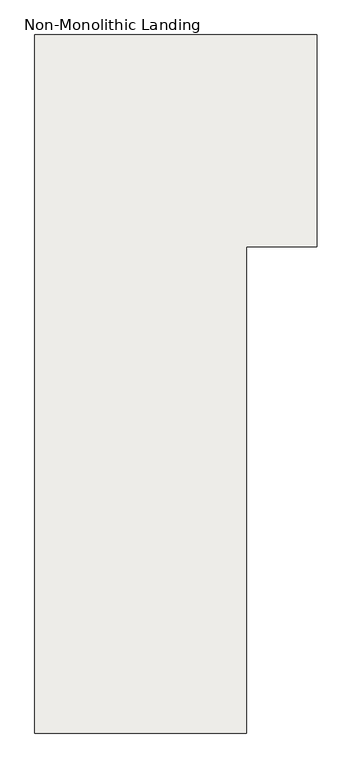
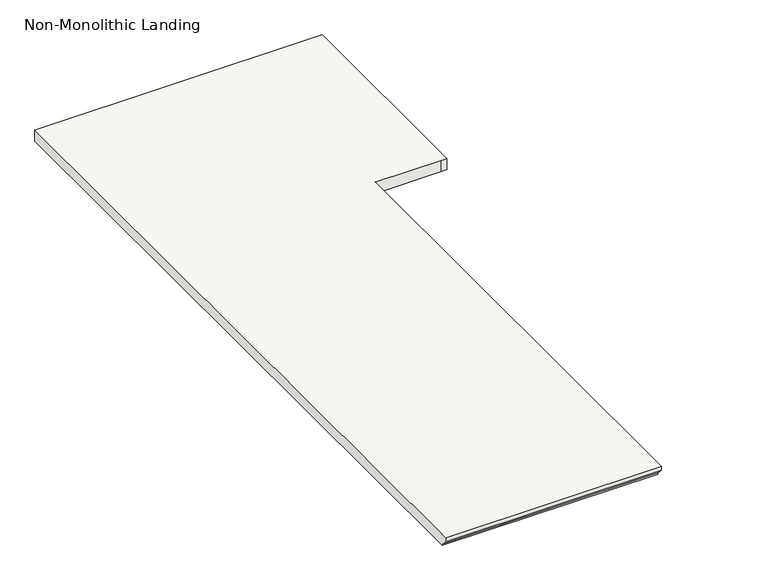
"""IFC4 building model written with IfcOpenShell, lengths in millimetres: slab geometry, Non-Monolithic Landing."""

from ifc_helpers import new_model, si_unit, origin, place, context, project, spatial, faceted_brep, source, transform, mapped, element, save


def non_monolithic_landing_d9f9278d(model_context):
    return source(origin(), model_context, "Body", "Brep", [
        faceted_brep([(-8119.8823175, 5251.0635177, 2182.2833333), (-8119.8823175, 5251.0635177, 2201.3333333), (-9034.2823175, 5251.0635177, 2201.3333333), (-9034.2823175, 5251.0635177, 2182.2833333), (-8119.8823175, 5276.4635177, 2156.8833333), (-9034.2823175, 5276.4635177, 2156.8833333), (-8119.8823175, 7352.205876, 2201.3333333), (-7840.4823175, 7352.205876, 2201.3333333), (-7815.0823175, 7352.205876, 2201.3333333), (-7815.0823175, 8266.605876, 2201.3333333), (-7840.4823175, 8266.605876, 2201.3333333), (-9034.2823175, 8266.605876, 2201.3333333), (-8119.8823175, 5276.4635177, 2150.5333333), (-9034.2823175, 5276.4635177, 2150.5333333), (-9034.2823175, 8266.605876, 2150.5333333), (-7840.4823175, 8266.605876, 2150.5333333), (-7815.0823175, 8266.605876, 2150.5333333), (-7815.0823175, 7352.205876, 2150.5333333), (-7840.4823175, 7352.205876, 2150.5333333), (-8119.8823175, 7352.205876, 2150.5333333)], [[[0, 1, 2, 3]], [[4, 0, 3, 5]], [[6, 7, 8, 9, 10, 11, 2, 1]], [[12, 13, 14, 15, 16, 17, 18, 19]], [[13, 12, 4, 5]], [[6, 1, 0, 4, 12, 19]], [[7, 6, 19, 18]], [[8, 7, 18, 17]], [[9, 8, 17, 16]], [[10, 9, 16, 15]], [[11, 10, 15, 14]], [[2, 11, 14, 13, 5, 3]]]),
    ])


if __name__ == "__main__":
    model = new_model("IFC4")
    model_context = context("Model", 3, world=origin())
    ifc_project = project(units=[si_unit("LENGTHUNIT", "METRE", prefix="MILLI")], contexts=[model_context])
    site = spatial("IfcSite", under=ifc_project)
    building = spatial("IfcBuilding", under=site)
    placement = place(None, origin())
    non_monolithic_landing_shape = non_monolithic_landing_d9f9278d(model_context)
    element("IfcSlab", 1, ObjectType="Non-Monolithic Landing", at=placement, inside=building, context=model_context, shape_type="MappedRepresentation", body=[
        mapped(non_monolithic_landing_shape, transform((0.0, 0.0, 0.0), x_axis=(1.0, 0.0, 0.0), y_axis=(0.0, 1.0, 0.0), z_axis=(0.0, 0.0, 1.0))),
    ])
    save(model, "model.ifc")
